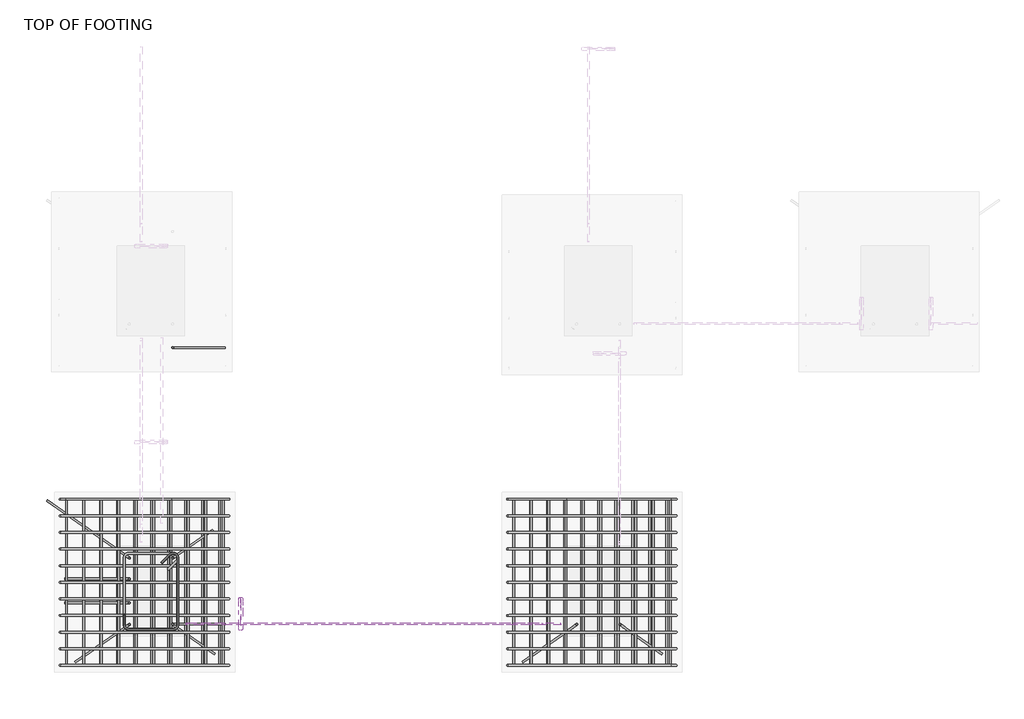
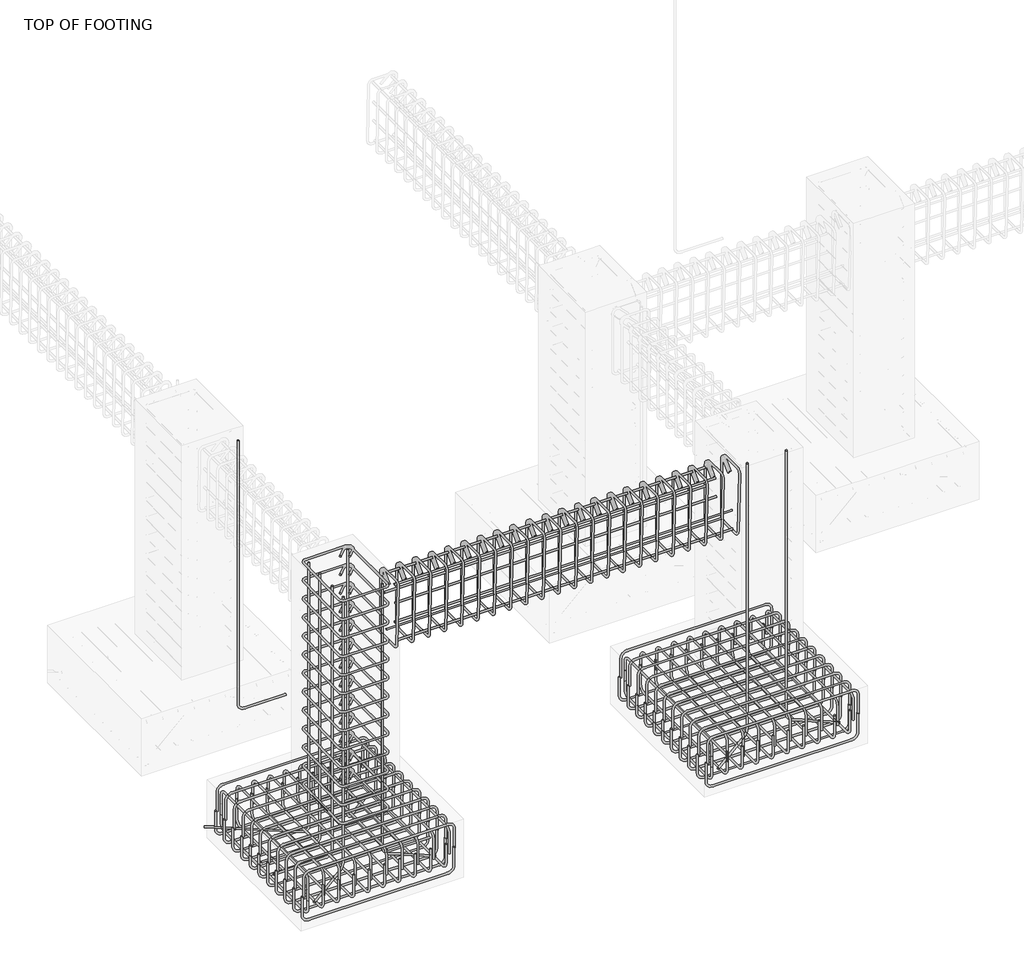
# One storey, part 2 of 17: 22 reinforcing bars.
"""IFC4 building model written with IfcOpenShell, lengths in millimetres."""

from ifc_helpers import new_model, si_unit, point, frame, origin, place, context, project, spatial, polyline, circle_curve, trimmed, segment, composite_curve, source, transform, mapped, element, save
from ifc_brep_helpers import swept_disk

model = new_model("IFC4")

# Units and contexts
model_context = context("Model", 3, world=origin())
ifc_project = project(units=[si_unit("LENGTHUNIT", "METRE", prefix="MILLI")], contexts=[model_context])

# Site, building, storey
site = spatial("IfcSite", under=ifc_project)
building = spatial("IfcBuilding", under=site)
storey = spatial("IfcBuildingStorey", under=building, Name="TOP OF FOOTING", Elevation=-1828.8)

# Reinforcing bars
placement = place(None, origin())
reinforcing_bar_shape = source(origin(), model_context, "Body", "SolidModel", [
    swept_disk(composite_curve([segment(polyline([(-2778.357124, -2320.8742842, -2051.4362487), (-2778.357124, -2320.8742842, -2198.7362487)]), True, "CONTINUOUS"), segment(trimmed(circle_curve(frame((-2824.707124, -2320.8742842, -2198.7362487), z_axis=(0.0, 1.0, 0.0), x_axis=(46.34999999999991, 0.0, 0.0)), 46.35), [point((-2778.357124, -2320.8742842, -2198.7362487))], [point((-2824.707124, -2320.8742842, -2245.0862487))], True, "CARTESIAN"), True, "CONTINUOUS"), segment(polyline([(-2824.707124, -2320.8742842, -2245.0862487), (-3850.0249485, -2320.8742842, -2245.0862487)]), True, "CONTINUOUS"), segment(trimmed(circle_curve(frame((-3850.0249485, -2320.8742842, -2198.7362487), z_axis=(0.0, 1.0, 0.0), x_axis=(0.0, 0.0, -46.34999999999991)), 46.35), [point((-3850.0249485, -2320.8742842, -2245.0862487))], [point((-3896.3749485, -2320.8742842, -2198.7362487))], True, "CARTESIAN"), True, "CONTINUOUS"), segment(polyline([(-3896.3749485, -2320.8742842, -2198.7362487), (-3896.3749485, -2320.8742842, -2051.4362487)]), True, "CONTINUOUS")], self_intersect=False), 6.35),
])
element("IfcReinforcingBar", 1, at=placement, inside=storey, context=model_context, shape_type="MappedRepresentation", body=[
    mapped(reinforcing_bar_shape, transform((0.0, 0.0, 0.0), x_axis=(1.0, 0.0, 0.0), y_axis=(0.0, 1.0, 0.0), z_axis=(0.0, 0.0, 1.0))),
    mapped(reinforcing_bar_shape, transform((0.0, -110.73, 0.0), x_axis=(1.0, 0.0, 0.0), y_axis=(0.0, 1.0, 0.0), z_axis=(0.0, 0.0, 1.0))),
    mapped(reinforcing_bar_shape, transform((0.0, -221.46, 0.0), x_axis=(1.0, 0.0, 0.0), y_axis=(0.0, 1.0, 0.0), z_axis=(0.0, 0.0, 1.0))),
    mapped(reinforcing_bar_shape, transform((0.0, -332.19, 0.0), x_axis=(1.0, 0.0, 0.0), y_axis=(0.0, 1.0, 0.0), z_axis=(0.0, 0.0, 1.0))),
    mapped(reinforcing_bar_shape, transform((0.0, -442.92, 0.0), x_axis=(1.0, 0.0, 0.0), y_axis=(0.0, 1.0, 0.0), z_axis=(0.0, 0.0, 1.0))),
    mapped(reinforcing_bar_shape, transform((0.0, -553.65, 0.0), x_axis=(1.0, 0.0, 0.0), y_axis=(0.0, 1.0, 0.0), z_axis=(0.0, 0.0, 1.0))),
    mapped(reinforcing_bar_shape, transform((0.0, -664.38, 0.0), x_axis=(1.0, 0.0, 0.0), y_axis=(0.0, 1.0, 0.0), z_axis=(0.0, 0.0, 1.0))),
    mapped(reinforcing_bar_shape, transform((0.0, -775.11, 0.0), x_axis=(1.0, 0.0, 0.0), y_axis=(0.0, 1.0, 0.0), z_axis=(0.0, 0.0, 1.0))),
    mapped(reinforcing_bar_shape, transform((0.0, -885.84, 0.0), x_axis=(1.0, 0.0, 0.0), y_axis=(0.0, 1.0, 0.0), z_axis=(0.0, 0.0, 1.0))),
    mapped(reinforcing_bar_shape, transform((0.0, -996.57, 0.0), x_axis=(1.0, 0.0, 0.0), y_axis=(0.0, 1.0, 0.0), z_axis=(0.0, 0.0, 1.0))),
    mapped(reinforcing_bar_shape, transform((0.0, -1107.3, 0.0), x_axis=(1.0, 0.0, 0.0), y_axis=(0.0, 1.0, 0.0), z_axis=(0.0, 0.0, 1.0))),
])
reinforcing_bar_2_shape = source(origin(), model_context, "Body", "SolidModel", [
    swept_disk(composite_curve([segment(polyline([(-3885.7112848, -2320.8742842, -2058.517229), (-3885.7112848, -2320.8742842, -1911.217229)]), True, "CONTINUOUS"), segment(trimmed(circle_curve(frame((-3839.3612848, -2320.8742842, -1911.217229), z_axis=(0.0, 1.0, 0.0), x_axis=(-46.350000000000364, 0.0, 0.0)), 46.35), [point((-3885.7112848, -2320.8742842, -1911.217229))], [point((-3839.3612848, -2320.8742842, -1864.867229))], True, "CARTESIAN"), True, "CONTINUOUS"), segment(polyline([(-3839.3612848, -2320.8742842, -1864.867229), (-2820.8048983, -2320.8742842, -1864.867229)]), True, "CONTINUOUS"), segment(trimmed(circle_curve(frame((-2820.8048983, -2320.8742842, -1911.217229), z_axis=(0.0, 1.0, 0.0), x_axis=(0.0, 0.0, 46.350000000000136)), 46.35), [point((-2820.8048983, -2320.8742842, -1864.867229))], [point((-2774.4548983, -2320.8742842, -1911.217229))], True, "CARTESIAN"), True, "CONTINUOUS"), segment(polyline([(-2774.4548983, -2320.8742842, -1911.217229), (-2774.4548983, -2320.8742842, -2058.517229)]), True, "CONTINUOUS")], self_intersect=False), 6.35),
])
element("IfcReinforcingBar", 2, at=placement, inside=storey, context=model_context, shape_type="MappedRepresentation", body=[
    mapped(reinforcing_bar_2_shape, transform((0.0, 0.0, 0.0), x_axis=(1.0, 0.0, 0.0), y_axis=(0.0, 1.0, 0.0), z_axis=(0.0, 0.0, 1.0))),
    mapped(reinforcing_bar_2_shape, transform((0.0, -110.73, 0.0), x_axis=(1.0, 0.0, 0.0), y_axis=(0.0, 1.0, 0.0), z_axis=(0.0, 0.0, 1.0))),
    mapped(reinforcing_bar_2_shape, transform((0.0, -221.46, 0.0), x_axis=(1.0, 0.0, 0.0), y_axis=(0.0, 1.0, 0.0), z_axis=(0.0, 0.0, 1.0))),
    mapped(reinforcing_bar_2_shape, transform((0.0, -332.19, 0.0), x_axis=(1.0, 0.0, 0.0), y_axis=(0.0, 1.0, 0.0), z_axis=(0.0, 0.0, 1.0))),
    mapped(reinforcing_bar_2_shape, transform((0.0, -442.92, 0.0), x_axis=(1.0, 0.0, 0.0), y_axis=(0.0, 1.0, 0.0), z_axis=(0.0, 0.0, 1.0))),
    mapped(reinforcing_bar_2_shape, transform((0.0, -553.65, 0.0), x_axis=(1.0, 0.0, 0.0), y_axis=(0.0, 1.0, 0.0), z_axis=(0.0, 0.0, 1.0))),
    mapped(reinforcing_bar_2_shape, transform((0.0, -664.38, 0.0), x_axis=(1.0, 0.0, 0.0), y_axis=(0.0, 1.0, 0.0), z_axis=(0.0, 0.0, 1.0))),
    mapped(reinforcing_bar_2_shape, transform((0.0, -775.11, 0.0), x_axis=(1.0, 0.0, 0.0), y_axis=(0.0, 1.0, 0.0), z_axis=(0.0, 0.0, 1.0))),
    mapped(reinforcing_bar_2_shape, transform((0.0, -885.84, 0.0), x_axis=(1.0, 0.0, 0.0), y_axis=(0.0, 1.0, 0.0), z_axis=(0.0, 0.0, 1.0))),
    mapped(reinforcing_bar_2_shape, transform((0.0, -996.57, 0.0), x_axis=(1.0, 0.0, 0.0), y_axis=(0.0, 1.0, 0.0), z_axis=(0.0, 0.0, 1.0))),
    mapped(reinforcing_bar_2_shape, transform((0.0, -1107.3, 0.0), x_axis=(1.0, 0.0, 0.0), y_axis=(0.0, 1.0, 0.0), z_axis=(0.0, 0.0, 1.0))),
])
reinforcing_bar_3_shape = source(origin(), model_context, "Body", "SolidModel", [
    swept_disk(composite_curve([segment(polyline([(-2811.4466034, -2320.8742842, -2093.0974099), (-2811.4466034, -2320.8742842, -1945.7974099)]), True, "CONTINUOUS"), segment(trimmed(circle_curve(frame((-2811.4466034, -2367.2242842, -1945.7974099), z_axis=(1.0, 0.0, 0.0), x_axis=(0.0, 46.34999999999991, 0.0)), 46.35), [point((-2811.4466034, -2320.8742842, -1945.7974099))], [point((-2811.4466034, -2367.2242842, -1899.4474099))], True, "CARTESIAN"), True, "CONTINUOUS"), segment(polyline([(-2811.4466034, -2367.2242842, -1899.4474099), (-2811.4466034, -3381.8242842, -1899.4474099)]), True, "CONTINUOUS"), segment(trimmed(circle_curve(frame((-2811.4466034, -3381.8242842, -1945.7974099), z_axis=(1.0, 0.0, 0.0), x_axis=(0.0, 0.0, 46.350000000000136)), 46.35), [point((-2811.4466034, -3381.8242842, -1899.4474099))], [point((-2811.4466034, -3428.1742842, -1945.7974099))], True, "CARTESIAN"), True, "CONTINUOUS"), segment(polyline([(-2811.4466034, -3428.1742842, -1945.7974099), (-2811.4466034, -3428.1742842, -2093.0974099)]), True, "CONTINUOUS")], self_intersect=False), 6.35),
])
element("IfcReinforcingBar", 3, at=placement, inside=storey, context=model_context, shape_type="MappedRepresentation", body=[
    mapped(reinforcing_bar_3_shape, transform((0.0, 0.0, 0.0), x_axis=(1.0, 0.0, 0.0), y_axis=(0.0, 1.0, 0.0), z_axis=(0.0, 0.0, 1.0))),
    mapped(reinforcing_bar_3_shape, transform((-115.9606781, 0.0, 0.0), x_axis=(1.0, 0.0, 0.0), y_axis=(0.0, 1.0, 0.0), z_axis=(0.0, 0.0, 1.0))),
    mapped(reinforcing_bar_3_shape, transform((-231.9213561, 0.0, 0.0), x_axis=(1.0, 0.0, 0.0), y_axis=(0.0, 1.0, 0.0), z_axis=(0.0, 0.0, 1.0))),
    mapped(reinforcing_bar_3_shape, transform((-347.8820342, 0.0, 0.0), x_axis=(1.0, 0.0, 0.0), y_axis=(0.0, 1.0, 0.0), z_axis=(0.0, 0.0, 1.0))),
    mapped(reinforcing_bar_3_shape, transform((-463.8427123, 0.0, 0.0), x_axis=(1.0, 0.0, 0.0), y_axis=(0.0, 1.0, 0.0), z_axis=(0.0, 0.0, 1.0))),
    mapped(reinforcing_bar_3_shape, transform((-579.8033904, 0.0, 0.0), x_axis=(1.0, 0.0, 0.0), y_axis=(0.0, 1.0, 0.0), z_axis=(0.0, 0.0, 1.0))),
    mapped(reinforcing_bar_3_shape, transform((-695.7640684, 0.0, 0.0), x_axis=(1.0, 0.0, 0.0), y_axis=(0.0, 1.0, 0.0), z_axis=(0.0, 0.0, 1.0))),
    mapped(reinforcing_bar_3_shape, transform((-811.7247465, 0.0, 0.0), x_axis=(1.0, 0.0, 0.0), y_axis=(0.0, 1.0, 0.0), z_axis=(0.0, 0.0, 1.0))),
    mapped(reinforcing_bar_3_shape, transform((-927.6854246, 0.0, 0.0), x_axis=(1.0, 0.0, 0.0), y_axis=(0.0, 1.0, 0.0), z_axis=(0.0, 0.0, 1.0))),
    mapped(reinforcing_bar_3_shape, transform((-1043.6461027, 0.0, 0.0), x_axis=(1.0, 0.0, 0.0), y_axis=(0.0, 1.0, 0.0), z_axis=(0.0, 0.0, 1.0))),
])
reinforcing_bar_4_shape = source(origin(), model_context, "Body", "SolidModel", [
    swept_disk(composite_curve([segment(polyline([(-3855.092706, -2320.8742842, -2009.4698822), (-3855.092706, -2320.8742842, -2156.7698822)]), True, "CONTINUOUS"), segment(trimmed(circle_curve(frame((-3855.092706, -2367.2242842, -2156.7698822), z_axis=(-1.0, 0.0, 0.0), x_axis=(0.0, 46.34999999999991, 0.0)), 46.35), [point((-3855.092706, -2320.8742842, -2156.7698822))], [point((-3855.092706, -2367.2242842, -2203.1198822))], True, "CARTESIAN"), True, "CONTINUOUS"), segment(polyline([(-3855.092706, -2367.2242842, -2203.1198822), (-3855.092706, -3381.8242842, -2203.1198822)]), True, "CONTINUOUS"), segment(trimmed(circle_curve(frame((-3855.092706, -3381.8242842, -2156.7698822), z_axis=(-1.0, 0.0, 0.0), x_axis=(0.0, 0.0, -46.34999999999991)), 46.35), [point((-3855.092706, -3381.8242842, -2203.1198822))], [point((-3855.092706, -3428.1742842, -2156.7698822))], True, "CARTESIAN"), True, "CONTINUOUS"), segment(polyline([(-3855.092706, -3428.1742842, -2156.7698822), (-3855.092706, -3428.1742842, -2009.4698822)]), True, "CONTINUOUS")], self_intersect=False), 6.35),
])
element("IfcReinforcingBar", 4, at=placement, inside=storey, context=model_context, shape_type="MappedRepresentation", body=[
    mapped(reinforcing_bar_4_shape, transform((0.0, 0.0, 0.0), x_axis=(1.0, 0.0, 0.0), y_axis=(0.0, 1.0, 0.0), z_axis=(0.0, 0.0, 1.0))),
    mapped(reinforcing_bar_4_shape, transform((113.1523491, 0.0, 0.0), x_axis=(1.0, 0.0, 0.0), y_axis=(0.0, 1.0, 0.0), z_axis=(0.0, 0.0, 1.0))),
    mapped(reinforcing_bar_4_shape, transform((226.3046983, 0.0, 0.0), x_axis=(1.0, 0.0, 0.0), y_axis=(0.0, 1.0, 0.0), z_axis=(0.0, 0.0, 1.0))),
    mapped(reinforcing_bar_4_shape, transform((339.4570474, 0.0, 0.0), x_axis=(1.0, 0.0, 0.0), y_axis=(0.0, 1.0, 0.0), z_axis=(0.0, 0.0, 1.0))),
    mapped(reinforcing_bar_4_shape, transform((452.6093966, 0.0, 0.0), x_axis=(1.0, 0.0, 0.0), y_axis=(0.0, 1.0, 0.0), z_axis=(0.0, 0.0, 1.0))),
    mapped(reinforcing_bar_4_shape, transform((565.7617457, 0.0, 0.0), x_axis=(1.0, 0.0, 0.0), y_axis=(0.0, 1.0, 0.0), z_axis=(0.0, 0.0, 1.0))),
    mapped(reinforcing_bar_4_shape, transform((678.9140949, 0.0, 0.0), x_axis=(1.0, 0.0, 0.0), y_axis=(0.0, 1.0, 0.0), z_axis=(0.0, 0.0, 1.0))),
    mapped(reinforcing_bar_4_shape, transform((792.066444, 0.0, 0.0), x_axis=(1.0, 0.0, 0.0), y_axis=(0.0, 1.0, 0.0), z_axis=(0.0, 0.0, 1.0))),
    mapped(reinforcing_bar_4_shape, transform((905.2187932, 0.0, 0.0), x_axis=(1.0, 0.0, 0.0), y_axis=(0.0, 1.0, 0.0), z_axis=(0.0, 0.0, 1.0))),
    mapped(reinforcing_bar_4_shape, transform((1018.3711423, 0.0, 0.0), x_axis=(1.0, 0.0, 0.0), y_axis=(0.0, 1.0, 0.0), z_axis=(0.0, 0.0, 1.0))),
])
reinforcing_bar_5_shape = source(origin(), model_context, "Body", "SolidModel", [
    swept_disk(composite_curve([segment(polyline([(199.2830257, -2320.8742842, -2051.4362487), (199.2830257, -2320.8742842, -2198.7362487)]), True, "CONTINUOUS"), segment(trimmed(circle_curve(frame((152.9330257, -2320.8742842, -2198.7362487), z_axis=(0.0, 1.0, 0.0), x_axis=(46.349999999999994, 0.0, 0.0)), 46.35), [point((199.2830257, -2320.8742842, -2198.7362487))], [point((152.9330257, -2320.8742842, -2245.0862487))], True, "CARTESIAN"), True, "CONTINUOUS"), segment(polyline([(152.9330257, -2320.8742842, -2245.0862487), (-872.3847988, -2320.8742842, -2245.0862487)]), True, "CONTINUOUS"), segment(trimmed(circle_curve(frame((-872.3847988, -2320.8742842, -2198.7362487), z_axis=(0.0, 1.0, 0.0), x_axis=(0.0, 0.0, -46.34999999999991)), 46.35), [point((-872.3847988, -2320.8742842, -2245.0862487))], [point((-918.7347988, -2320.8742842, -2198.7362487))], True, "CARTESIAN"), True, "CONTINUOUS"), segment(polyline([(-918.7347988, -2320.8742842, -2198.7362487), (-918.7347988, -2320.8742842, -2051.4362487)]), True, "CONTINUOUS")], self_intersect=False), 6.35),
])
element("IfcReinforcingBar", 5, at=placement, inside=storey, context=model_context, shape_type="MappedRepresentation", body=[
    mapped(reinforcing_bar_5_shape, transform((0.0, 0.0, 0.0), x_axis=(1.0, 0.0, 0.0), y_axis=(0.0, 1.0, 0.0), z_axis=(0.0, 0.0, 1.0))),
    mapped(reinforcing_bar_5_shape, transform((0.0, -110.73, 0.0), x_axis=(1.0, 0.0, 0.0), y_axis=(0.0, 1.0, 0.0), z_axis=(0.0, 0.0, 1.0))),
    mapped(reinforcing_bar_5_shape, transform((0.0, -221.46, 0.0), x_axis=(1.0, 0.0, 0.0), y_axis=(0.0, 1.0, 0.0), z_axis=(0.0, 0.0, 1.0))),
    mapped(reinforcing_bar_5_shape, transform((0.0, -332.19, 0.0), x_axis=(1.0, 0.0, 0.0), y_axis=(0.0, 1.0, 0.0), z_axis=(0.0, 0.0, 1.0))),
    mapped(reinforcing_bar_5_shape, transform((0.0, -442.92, 0.0), x_axis=(1.0, 0.0, 0.0), y_axis=(0.0, 1.0, 0.0), z_axis=(0.0, 0.0, 1.0))),
    mapped(reinforcing_bar_5_shape, transform((0.0, -553.65, 0.0), x_axis=(1.0, 0.0, 0.0), y_axis=(0.0, 1.0, 0.0), z_axis=(0.0, 0.0, 1.0))),
    mapped(reinforcing_bar_5_shape, transform((0.0, -664.38, 0.0), x_axis=(1.0, 0.0, 0.0), y_axis=(0.0, 1.0, 0.0), z_axis=(0.0, 0.0, 1.0))),
    mapped(reinforcing_bar_5_shape, transform((0.0, -775.11, 0.0), x_axis=(1.0, 0.0, 0.0), y_axis=(0.0, 1.0, 0.0), z_axis=(0.0, 0.0, 1.0))),
    mapped(reinforcing_bar_5_shape, transform((0.0, -885.84, 0.0), x_axis=(1.0, 0.0, 0.0), y_axis=(0.0, 1.0, 0.0), z_axis=(0.0, 0.0, 1.0))),
    mapped(reinforcing_bar_5_shape, transform((0.0, -996.57, 0.0), x_axis=(1.0, 0.0, 0.0), y_axis=(0.0, 1.0, 0.0), z_axis=(0.0, 0.0, 1.0))),
    mapped(reinforcing_bar_5_shape, transform((0.0, -1107.3, 0.0), x_axis=(1.0, 0.0, 0.0), y_axis=(0.0, 1.0, 0.0), z_axis=(0.0, 0.0, 1.0))),
])
reinforcing_bar_6_shape = source(origin(), model_context, "Body", "SolidModel", [
    swept_disk(composite_curve([segment(polyline([(-908.0711351, -2320.8742842, -2058.517229), (-908.0711351, -2320.8742842, -1911.217229)]), True, "CONTINUOUS"), segment(trimmed(circle_curve(frame((-861.7211351, -2320.8742842, -1911.217229), z_axis=(0.0, 1.0, 0.0), x_axis=(-46.35000000000002, 0.0, 0.0)), 46.35), [point((-908.0711351, -2320.8742842, -1911.217229))], [point((-861.7211351, -2320.8742842, -1864.867229))], True, "CARTESIAN"), True, "CONTINUOUS"), segment(polyline([(-861.7211351, -2320.8742842, -1864.867229), (156.8352514, -2320.8742842, -1864.867229)]), True, "CONTINUOUS"), segment(trimmed(circle_curve(frame((156.8352514, -2320.8742842, -1911.217229), z_axis=(0.0, 1.0, 0.0), x_axis=(0.0, 0.0, 46.350000000000136)), 46.35), [point((156.8352514, -2320.8742842, -1864.867229))], [point((203.1852514, -2320.8742842, -1911.217229))], True, "CARTESIAN"), True, "CONTINUOUS"), segment(polyline([(203.1852514, -2320.8742842, -1911.217229), (203.1852514, -2320.8742842, -2058.517229)]), True, "CONTINUOUS")], self_intersect=False), 6.35),
])
element("IfcReinforcingBar", 6, at=placement, inside=storey, context=model_context, shape_type="MappedRepresentation", body=[
    mapped(reinforcing_bar_6_shape, transform((0.0, 0.0, 0.0), x_axis=(1.0, 0.0, 0.0), y_axis=(0.0, 1.0, 0.0), z_axis=(0.0, 0.0, 1.0))),
    mapped(reinforcing_bar_6_shape, transform((0.0, -110.73, 0.0), x_axis=(1.0, 0.0, 0.0), y_axis=(0.0, 1.0, 0.0), z_axis=(0.0, 0.0, 1.0))),
    mapped(reinforcing_bar_6_shape, transform((0.0, -221.46, 0.0), x_axis=(1.0, 0.0, 0.0), y_axis=(0.0, 1.0, 0.0), z_axis=(0.0, 0.0, 1.0))),
    mapped(reinforcing_bar_6_shape, transform((0.0, -332.19, 0.0), x_axis=(1.0, 0.0, 0.0), y_axis=(0.0, 1.0, 0.0), z_axis=(0.0, 0.0, 1.0))),
    mapped(reinforcing_bar_6_shape, transform((0.0, -442.92, 0.0), x_axis=(1.0, 0.0, 0.0), y_axis=(0.0, 1.0, 0.0), z_axis=(0.0, 0.0, 1.0))),
    mapped(reinforcing_bar_6_shape, transform((0.0, -553.65, 0.0), x_axis=(1.0, 0.0, 0.0), y_axis=(0.0, 1.0, 0.0), z_axis=(0.0, 0.0, 1.0))),
    mapped(reinforcing_bar_6_shape, transform((0.0, -664.38, 0.0), x_axis=(1.0, 0.0, 0.0), y_axis=(0.0, 1.0, 0.0), z_axis=(0.0, 0.0, 1.0))),
    mapped(reinforcing_bar_6_shape, transform((0.0, -775.11, 0.0), x_axis=(1.0, 0.0, 0.0), y_axis=(0.0, 1.0, 0.0), z_axis=(0.0, 0.0, 1.0))),
    mapped(reinforcing_bar_6_shape, transform((0.0, -885.84, 0.0), x_axis=(1.0, 0.0, 0.0), y_axis=(0.0, 1.0, 0.0), z_axis=(0.0, 0.0, 1.0))),
    mapped(reinforcing_bar_6_shape, transform((0.0, -996.57, 0.0), x_axis=(1.0, 0.0, 0.0), y_axis=(0.0, 1.0, 0.0), z_axis=(0.0, 0.0, 1.0))),
    mapped(reinforcing_bar_6_shape, transform((0.0, -1107.3, 0.0), x_axis=(1.0, 0.0, 0.0), y_axis=(0.0, 1.0, 0.0), z_axis=(0.0, 0.0, 1.0))),
])
reinforcing_bar_7_shape = source(origin(), model_context, "Body", "SolidModel", [
    swept_disk(composite_curve([segment(polyline([(166.1935463, -2320.8742842, -2093.0974099), (166.1935463, -2320.8742842, -1945.7974099)]), True, "CONTINUOUS"), segment(trimmed(circle_curve(frame((166.1935463, -2367.2242842, -1945.7974099), z_axis=(1.0, 0.0, 0.0), x_axis=(0.0, 46.34999999999991, 0.0)), 46.35), [point((166.1935463, -2320.8742842, -1945.7974099))], [point((166.1935463, -2367.2242842, -1899.4474099))], True, "CARTESIAN"), True, "CONTINUOUS"), segment(polyline([(166.1935463, -2367.2242842, -1899.4474099), (166.1935463, -3381.8242842, -1899.4474099)]), True, "CONTINUOUS"), segment(trimmed(circle_curve(frame((166.1935463, -3381.8242842, -1945.7974099), z_axis=(1.0, 0.0, 0.0), x_axis=(0.0, 0.0, 46.350000000000136)), 46.35), [point((166.1935463, -3381.8242842, -1899.4474099))], [point((166.1935463, -3428.1742842, -1945.7974099))], True, "CARTESIAN"), True, "CONTINUOUS"), segment(polyline([(166.1935463, -3428.1742842, -1945.7974099), (166.1935463, -3428.1742842, -2093.0974099)]), True, "CONTINUOUS")], self_intersect=False), 6.35),
])
element("IfcReinforcingBar", 7, at=placement, inside=storey, context=model_context, shape_type="MappedRepresentation", body=[
    mapped(reinforcing_bar_7_shape, transform((0.0, 0.0, 0.0), x_axis=(1.0, 0.0, 0.0), y_axis=(0.0, 1.0, 0.0), z_axis=(0.0, 0.0, 1.0))),
    mapped(reinforcing_bar_7_shape, transform((-115.9606781, 0.0, 0.0), x_axis=(1.0, 0.0, 0.0), y_axis=(0.0, 1.0, 0.0), z_axis=(0.0, 0.0, 1.0))),
    mapped(reinforcing_bar_7_shape, transform((-231.9213561, 0.0, 0.0), x_axis=(1.0, 0.0, 0.0), y_axis=(0.0, 1.0, 0.0), z_axis=(0.0, 0.0, 1.0))),
    mapped(reinforcing_bar_7_shape, transform((-347.8820342, 0.0, 0.0), x_axis=(1.0, 0.0, 0.0), y_axis=(0.0, 1.0, 0.0), z_axis=(0.0, 0.0, 1.0))),
    mapped(reinforcing_bar_7_shape, transform((-463.8427123, 0.0, 0.0), x_axis=(1.0, 0.0, 0.0), y_axis=(0.0, 1.0, 0.0), z_axis=(0.0, 0.0, 1.0))),
    mapped(reinforcing_bar_7_shape, transform((-579.8033904, 0.0, 0.0), x_axis=(1.0, 0.0, 0.0), y_axis=(0.0, 1.0, 0.0), z_axis=(0.0, 0.0, 1.0))),
    mapped(reinforcing_bar_7_shape, transform((-695.7640684, 0.0, 0.0), x_axis=(1.0, 0.0, 0.0), y_axis=(0.0, 1.0, 0.0), z_axis=(0.0, 0.0, 1.0))),
    mapped(reinforcing_bar_7_shape, transform((-811.7247465, 0.0, 0.0), x_axis=(1.0, 0.0, 0.0), y_axis=(0.0, 1.0, 0.0), z_axis=(0.0, 0.0, 1.0))),
    mapped(reinforcing_bar_7_shape, transform((-927.6854246, 0.0, 0.0), x_axis=(1.0, 0.0, 0.0), y_axis=(0.0, 1.0, 0.0), z_axis=(0.0, 0.0, 1.0))),
    mapped(reinforcing_bar_7_shape, transform((-1043.6461027, 0.0, 0.0), x_axis=(1.0, 0.0, 0.0), y_axis=(0.0, 1.0, 0.0), z_axis=(0.0, 0.0, 1.0))),
])
reinforcing_bar_8_shape = source(origin(), model_context, "Body", "SolidModel", [
    swept_disk(composite_curve([segment(polyline([(-877.4525564, -2320.8742842, -2009.4698822), (-877.4525564, -2320.8742842, -2156.7698822)]), True, "CONTINUOUS"), segment(trimmed(circle_curve(frame((-877.4525564, -2367.2242842, -2156.7698822), z_axis=(-1.0, 0.0, 0.0), x_axis=(0.0, 46.34999999999991, 0.0)), 46.35), [point((-877.4525564, -2320.8742842, -2156.7698822))], [point((-877.4525564, -2367.2242842, -2203.1198822))], True, "CARTESIAN"), True, "CONTINUOUS"), segment(polyline([(-877.4525564, -2367.2242842, -2203.1198822), (-877.4525564, -3381.8242842, -2203.1198822)]), True, "CONTINUOUS"), segment(trimmed(circle_curve(frame((-877.4525564, -3381.8242842, -2156.7698822), z_axis=(-1.0, 0.0, 0.0), x_axis=(0.0, 0.0, -46.34999999999991)), 46.35), [point((-877.4525564, -3381.8242842, -2203.1198822))], [point((-877.4525564, -3428.1742842, -2156.7698822))], True, "CARTESIAN"), True, "CONTINUOUS"), segment(polyline([(-877.4525564, -3428.1742842, -2156.7698822), (-877.4525564, -3428.1742842, -2009.4698822)]), True, "CONTINUOUS")], self_intersect=False), 6.35),
])
element("IfcReinforcingBar", 8, at=placement, inside=storey, context=model_context, shape_type="MappedRepresentation", body=[
    mapped(reinforcing_bar_8_shape, transform((0.0, 0.0, 0.0), x_axis=(1.0, 0.0, 0.0), y_axis=(0.0, 1.0, 0.0), z_axis=(0.0, 0.0, 1.0))),
    mapped(reinforcing_bar_8_shape, transform((113.1523491, 0.0, 0.0), x_axis=(1.0, 0.0, 0.0), y_axis=(0.0, 1.0, 0.0), z_axis=(0.0, 0.0, 1.0))),
    mapped(reinforcing_bar_8_shape, transform((226.3046983, 0.0, 0.0), x_axis=(1.0, 0.0, 0.0), y_axis=(0.0, 1.0, 0.0), z_axis=(0.0, 0.0, 1.0))),
    mapped(reinforcing_bar_8_shape, transform((339.4570474, 0.0, 0.0), x_axis=(1.0, 0.0, 0.0), y_axis=(0.0, 1.0, 0.0), z_axis=(0.0, 0.0, 1.0))),
    mapped(reinforcing_bar_8_shape, transform((452.6093966, 0.0, 0.0), x_axis=(1.0, 0.0, 0.0), y_axis=(0.0, 1.0, 0.0), z_axis=(0.0, 0.0, 1.0))),
    mapped(reinforcing_bar_8_shape, transform((565.7617457, 0.0, 0.0), x_axis=(1.0, 0.0, 0.0), y_axis=(0.0, 1.0, 0.0), z_axis=(0.0, 0.0, 1.0))),
    mapped(reinforcing_bar_8_shape, transform((678.9140949, 0.0, 0.0), x_axis=(1.0, 0.0, 0.0), y_axis=(0.0, 1.0, 0.0), z_axis=(0.0, 0.0, 1.0))),
    mapped(reinforcing_bar_8_shape, transform((792.066444, 0.0, 0.0), x_axis=(1.0, 0.0, 0.0), y_axis=(0.0, 1.0, 0.0), z_axis=(0.0, 0.0, 1.0))),
    mapped(reinforcing_bar_8_shape, transform((905.2187932, 0.0, 0.0), x_axis=(1.0, 0.0, 0.0), y_axis=(0.0, 1.0, 0.0), z_axis=(0.0, 0.0, 1.0))),
    mapped(reinforcing_bar_8_shape, transform((1018.3711423, 0.0, 0.0), x_axis=(1.0, 0.0, 0.0), y_axis=(0.0, 1.0, 0.0), z_axis=(0.0, 0.0, 1.0))),
])
reinforcing_bar_9_shape = source(origin(), model_context, "Body", "SolidModel", [
    swept_disk(composite_curve([segment(polyline([(-3222.6184845, -2745.8000495, -46.35), (-3166.8749216, -2690.0564866, -46.35)]), True, "CONTINUOUS"), segment(trimmed(circle_curve(frame((-3144.707124, -2712.2242842, -46.35), z_axis=(0.0, 0.0, -1.0), x_axis=(-22.167797600000085, 22.167797600000085, 0.0)), 31.35), [point((-3166.8749216, -2690.0564866, -46.35))], [point((-3113.357124, -2712.2242842, -46.35))], True, "CARTESIAN"), True, "CONTINUOUS"), segment(polyline([(-3113.357124, -2712.2242842, -46.35), (-3113.357124, -3156.8242842, -46.35)]), True, "CONTINUOUS"), segment(trimmed(circle_curve(frame((-3144.707124, -3156.8242842, -46.35), z_axis=(0.0, 0.0, -1.0), x_axis=(31.34999999999991, 0.0, 0.0)), 31.35), [point((-3113.357124, -3156.8242842, -46.35))], [point((-3144.707124, -3188.1742842, -46.35))], True, "CARTESIAN"), True, "CONTINUOUS"), segment(polyline([(-3144.707124, -3188.1742842, -46.35), (-3439.307124, -3188.1742842, -46.35)]), True, "CONTINUOUS"), segment(trimmed(circle_curve(frame((-3439.307124, -3156.8341035, -45.5654144), z_axis=(0.0, 0.025026655153786343, -0.9996867842138424), x_axis=(0.0, -31.34018070000002, -0.7845855999999998)), 31.35), [point((-3439.307124, -3188.1742842, -46.35))], [point((-3470.657124, -3156.8341035, -45.5654144))], True, "CARTESIAN"), True, "CONTINUOUS"), segment(polyline([(-3470.657124, -3156.8341035, -45.5654144), (-3470.657124, -2712.2144649, -34.4345856)]), True, "CONTINUOUS"), segment(trimmed(circle_curve(frame((-3439.307124, -2712.2144649, -34.4345856), z_axis=(0.0, 0.025026655153786343, -0.9996867842138424), x_axis=(-31.34999999999991, 0.0, 0.0)), 31.35), [point((-3470.657124, -2712.2144649, -34.4345856))], [point((-3439.307124, -2680.8742842, -33.65))], True, "CARTESIAN"), True, "CONTINUOUS"), segment(polyline([(-3439.307124, -2680.8742842, -33.65), (-3144.707124, -2680.8742842, -33.65)]), True, "CONTINUOUS"), segment(trimmed(circle_curve(frame((-3144.707124, -2712.2242842, -33.65), z_axis=(0.0, 0.0, -1.0), x_axis=(0.0, 31.34999999999991, 0.0)), 31.35), [point((-3144.707124, -2680.8742842, -33.65))], [point((-3122.5393264, -2734.3920818, -33.65))], True, "CARTESIAN"), True, "CONTINUOUS"), segment(polyline([(-3122.5393264, -2734.3920818, -33.65), (-3178.2828893, -2790.1356447, -33.65)]), True, "CONTINUOUS")], self_intersect=False), 6.35),
])
element("IfcReinforcingBar", 9, at=placement, inside=storey, context=model_context, shape_type="MappedRepresentation", body=[
    mapped(reinforcing_bar_9_shape, transform((0.0, 0.0, 0.0), x_axis=(1.0, 0.0, 0.0), y_axis=(0.0, 1.0, 0.0), z_axis=(0.0, 0.0, 1.0))),
    mapped(reinforcing_bar_9_shape, transform((0.0, 0.0, -144.675), x_axis=(1.0, 0.0, 0.0), y_axis=(0.0, 1.0, 0.0), z_axis=(0.0, 0.0, 1.0))),
    mapped(reinforcing_bar_9_shape, transform((0.0, 0.0, -289.35), x_axis=(1.0, 0.0, 0.0), y_axis=(0.0, 1.0, 0.0), z_axis=(0.0, 0.0, 1.0))),
    mapped(reinforcing_bar_9_shape, transform((0.0, 0.0, -434.025), x_axis=(1.0, 0.0, 0.0), y_axis=(0.0, 1.0, 0.0), z_axis=(0.0, 0.0, 1.0))),
    mapped(reinforcing_bar_9_shape, transform((0.0, 0.0, -578.7), x_axis=(1.0, 0.0, 0.0), y_axis=(0.0, 1.0, 0.0), z_axis=(0.0, 0.0, 1.0))),
    mapped(reinforcing_bar_9_shape, transform((0.0, 0.0, -723.375), x_axis=(1.0, 0.0, 0.0), y_axis=(0.0, 1.0, 0.0), z_axis=(0.0, 0.0, 1.0))),
    mapped(reinforcing_bar_9_shape, transform((0.0, 0.0, -868.05), x_axis=(1.0, 0.0, 0.0), y_axis=(0.0, 1.0, 0.0), z_axis=(0.0, 0.0, 1.0))),
    mapped(reinforcing_bar_9_shape, transform((0.0, 0.0, -1012.725), x_axis=(1.0, 0.0, 0.0), y_axis=(0.0, 1.0, 0.0), z_axis=(0.0, 0.0, 1.0))),
    mapped(reinforcing_bar_9_shape, transform((0.0, 0.0, -1157.4), x_axis=(1.0, 0.0, 0.0), y_axis=(0.0, 1.0, 0.0), z_axis=(0.0, 0.0, 1.0))),
    mapped(reinforcing_bar_9_shape, transform((0.0, 0.0, -1302.075), x_axis=(1.0, 0.0, 0.0), y_axis=(0.0, 1.0, 0.0), z_axis=(0.0, 0.0, 1.0))),
    mapped(reinforcing_bar_9_shape, transform((0.0, 0.0, -1446.75), x_axis=(1.0, 0.0, 0.0), y_axis=(0.0, 1.0, 0.0), z_axis=(0.0, 0.0, 1.0))),
    mapped(reinforcing_bar_9_shape, transform((0.0, 0.0, -1591.425), x_axis=(1.0, 0.0, 0.0), y_axis=(0.0, 1.0, 0.0), z_axis=(0.0, 0.0, 1.0))),
    mapped(reinforcing_bar_9_shape, transform((0.0, 0.0, -1736.1), x_axis=(1.0, 0.0, 0.0), y_axis=(0.0, 1.0, 0.0), z_axis=(0.0, 0.0, 1.0))),
])
reinforcing_bar_10_shape = source(origin(), model_context, "Body", "SolidModel", [
    swept_disk(composite_curve([segment(polyline([(-3147.7427136, -3152.6310005, -40.0), (-3147.7427136, -3152.6310005, -2094.5391135)]), True, "CONTINUOUS"), segment(trimmed(circle_curve(frame((-3101.3927136, -3152.6310005, -2094.5391135), z_axis=(0.0, -1.0, 0.0), x_axis=(-46.34999999999991, 0.0, 0.0)), 46.35), [point((-3147.7427136, -3152.6310005, -2094.5391135))], [point((-3101.3927136, -3152.6310005, -2140.8891135))], True, "CARTESIAN"), True, "CONTINUOUS"), segment(polyline([(-3101.3927136, -3152.6310005, -2140.8891135), (-2797.6608063, -3152.6310005, -2140.8891135)]), True, "CONTINUOUS")], self_intersect=False), 6.35),
])
element("IfcReinforcingBar", 10, at=placement, inside=storey, context=model_context, shape_type="MappedRepresentation", body=[
    mapped(reinforcing_bar_10_shape, transform((0.0, 0.0, 0.0), x_axis=(1.0, 0.0, 0.0), y_axis=(0.0, 1.0, 0.0), z_axis=(0.0, 0.0, 1.0))),
    mapped(reinforcing_bar_10_shape, transform((0.0, 1840.7260472, 0.0), x_axis=(1.0, 0.0, 0.0), y_axis=(0.0, 1.0, 0.0), z_axis=(0.0, 0.0, 1.0))),
])
element("IfcReinforcingBar", 11, at=placement, inside=storey, context=model_context, shape_type="SolidModel", body=[
    swept_disk(composite_curve([segment(polyline([(-3147.7427136, -2713.5742842, -40.0), (-3147.7427136, -2713.5742842, -2094.5391135)]), True, "CONTINUOUS"), segment(trimmed(circle_curve(frame((-3109.7750164, -2686.9890164, -2094.5391135), z_axis=(0.5735764363510363, -0.8191520442889988, 0.0), x_axis=(-37.9676972000002, -26.58526780000011, 0.0)), 46.35), [point((-3147.7427136, -2713.5742842, -2094.5391135))], [point((-3109.7750164, -2686.9890164, -2140.8891135))], True, "CARTESIAN"), True, "CONTINUOUS"), segment(polyline([(-3109.7750164, -2686.9890164, -2140.8891135), (-2881.4249234, -2527.0965599, -2140.8891135)]), True, "CONTINUOUS")], self_intersect=False), 6.35),
])
element("IfcReinforcingBar", 12, at=placement, inside=storey, context=model_context, shape_type="SolidModel", body=[
    swept_disk(composite_curve([segment(polyline([(-3436.2715343, -2713.5742842, -40.0), (-3436.2715343, -2713.5742842, -2094.5391135)]), True, "CONTINUOUS"), segment(trimmed(circle_curve(frame((-3474.2392316, -2686.9890164, -2094.5391135), z_axis=(0.5735764363510419, 0.8191520442889948, 0.0), x_axis=(37.967697300000054, -26.58526780000011, 0.0)), 46.35), [point((-3436.2715343, -2713.5742842, -2094.5391135))], [point((-3474.2392316, -2686.9890164, -2140.8891135))], True, "CARTESIAN"), True, "CONTINUOUS"), segment(polyline([(-3474.2392316, -2686.9890164, -2140.8891135), (-3984.3116072, -2329.8324939, -2140.8891135)]), True, "CONTINUOUS")], self_intersect=False), 6.35),
])
element("IfcReinforcingBar", 13, at=placement, inside=storey, context=model_context, shape_type="SolidModel", body=[
    swept_disk(composite_curve([segment(polyline([(-3147.7427136, -3155.4742842, -40.0), (-3147.7427136, -3155.4742842, -2094.5391135)]), True, "CONTINUOUS"), segment(trimmed(circle_curve(frame((-3109.7750164, -3182.059552, -2094.5391135), z_axis=(-0.5735764363510363, -0.8191520442889988, 0.0), x_axis=(-37.9676972000002, 26.58526780000011, 0.0)), 46.35), [point((-3147.7427136, -3155.4742842, -2094.5391135))], [point((-3109.7750164, -3182.059552, -2140.8891135))], True, "CARTESIAN"), True, "CONTINUOUS"), segment(polyline([(-3109.7750164, -3182.059552, -2140.8891135), (-2868.2063218, -3351.207773, -2140.8891135)]), True, "CONTINUOUS")], self_intersect=False), 6.35),
])
element("IfcReinforcingBar", 14, at=placement, inside=storey, context=model_context, shape_type="SolidModel", body=[
    swept_disk(composite_curve([segment(polyline([(-3436.2715343, -3155.4742842, -40.0), (-3436.2715343, -3155.4742842, -2094.5391135)]), True, "CONTINUOUS"), segment(trimmed(circle_curve(frame((-3474.2392316, -3182.059552, -2094.5391135), z_axis=(-0.5735764363510419, 0.8191520442889948, 0.0), x_axis=(37.967697300000054, 26.58526780000011, 0.0)), 46.35), [point((-3436.2715343, -3155.4742842, -2094.5391135))], [point((-3474.2392316, -3182.059552, -2140.8891135))], True, "CARTESIAN"), True, "CONTINUOUS"), segment(polyline([(-3474.2392316, -3182.059552, -2140.8891135), (-3795.8079262, -3407.224376, -2140.8891135)]), True, "CONTINUOUS")], self_intersect=False), 6.35),
])
reinforcing_bar_11_shape = source(origin(), model_context, "Body", "SolidModel", [
    swept_disk(composite_curve([segment(polyline([(-3436.2715343, -2852.6310005, -40.0), (-3436.2715343, -2852.6310005, -2094.5391135)]), True, "CONTINUOUS"), segment(trimmed(circle_curve(frame((-3482.6215343, -2852.6310005, -2094.5391135), z_axis=(0.0, 1.0, 0.0), x_axis=(46.34999999999991, 0.0, 0.0)), 46.35), [point((-3436.2715343, -2852.6310005, -2094.5391135))], [point((-3482.6215343, -2852.6310005, -2140.8891135))], True, "CARTESIAN"), True, "CONTINUOUS"), segment(polyline([(-3482.6215343, -2852.6310005, -2140.8891135), (-3866.3534417, -2852.6310005, -2140.8891135)]), True, "CONTINUOUS")], self_intersect=False), 6.35),
])
element("IfcReinforcingBar", 15, at=placement, inside=storey, context=model_context, shape_type="MappedRepresentation", body=[
    mapped(reinforcing_bar_11_shape, transform((0.0, 0.0, 0.0), x_axis=(1.0, 0.0, 0.0), y_axis=(0.0, 1.0, 0.0), z_axis=(0.0, 0.0, 1.0))),
    mapped(reinforcing_bar_11_shape, transform((0.0, -159.2739528, 0.0), x_axis=(1.0, 0.0, 0.0), y_axis=(0.0, 1.0, 0.0), z_axis=(0.0, 0.0, 1.0))),
])
element("IfcReinforcingBar", 16, at=placement, inside=storey, context=model_context, shape_type="SolidModel", body=[
    swept_disk(composite_curve([segment(polyline([(-170.102564, -3155.4742842, -40.0), (-170.102564, -3155.4742842, -2094.5391135)]), True, "CONTINUOUS"), segment(trimmed(circle_curve(frame((-132.1348667, -3182.059552, -2094.5391135), z_axis=(-0.5735764363510363, -0.8191520442889988, 0.0), x_axis=(-37.9676973, 26.58526780000011, 0.0)), 46.35), [point((-170.102564, -3155.4742842, -2094.5391135))], [point((-132.1348667, -3182.059552, -2140.8891135))], True, "CARTESIAN"), True, "CONTINUOUS"), segment(polyline([(-132.1348667, -3182.059552, -2140.8891135), (109.4338279, -3351.207773, -2140.8891135)]), True, "CONTINUOUS")], self_intersect=False), 6.35),
])
element("IfcReinforcingBar", 17, at=placement, inside=storey, context=model_context, shape_type="SolidModel", body=[
    swept_disk(composite_curve([segment(polyline([(-458.6313847, -3155.4742842, -40.0), (-458.6313847, -3155.4742842, -2094.5391135)]), True, "CONTINUOUS"), segment(trimmed(circle_curve(frame((-496.5990819, -3182.059552, -2094.5391135), z_axis=(-0.5735764363510419, 0.8191520442889948, 0.0), x_axis=(37.967697199999975, 26.58526780000011, 0.0)), 46.35), [point((-458.6313847, -3155.4742842, -2094.5391135))], [point((-496.5990819, -3182.059552, -2140.8891135))], True, "CARTESIAN"), True, "CONTINUOUS"), segment(polyline([(-496.5990819, -3182.059552, -2140.8891135), (-818.1677765, -3407.224376, -2140.8891135)]), True, "CONTINUOUS")], self_intersect=False), 6.35),
])
reinforcing_bar_12_shape = source(origin(), model_context, "Body", "SolidModel", [
    swept_disk(composite_curve([segment(polyline([(-545.7169743, -3090.1356447, -111.2757654), (-545.7169743, -3034.3920818, -55.5322024)]), True, "CONTINUOUS"), segment(trimmed(circle_curve(frame((-545.7169743, -3012.2242842, -77.7), z_axis=(-1.0, 0.0, 0.0), x_axis=(0.0, -22.167797600000085, 22.1677976)), 31.35), [point((-545.7169743, -3034.3920818, -55.5322024))], [point((-545.7169743, -2980.8742842, -77.7))], True, "CARTESIAN"), True, "CONTINUOUS"), segment(polyline([(-545.7169743, -2980.8742842, -77.7), (-545.7169743, -2980.8742842, -522.3)]), True, "CONTINUOUS"), segment(trimmed(circle_curve(frame((-545.7169743, -3012.2242842, -522.3), z_axis=(-1.0, 0.0, 0.0), x_axis=(0.0, 31.34999999999991, 0.0)), 31.35), [point((-545.7169743, -2980.8742842, -522.3))], [point((-545.7169743, -3012.2242842, -553.65))], True, "CARTESIAN"), True, "CONTINUOUS"), segment(polyline([(-545.7169743, -3012.2242842, -553.65), (-545.7169743, -3156.8242842, -553.65)]), True, "CONTINUOUS"), segment(trimmed(circle_curve(frame((-544.9323887, -3156.8242842, -522.3098193), z_axis=(-0.9996867842138424, 0.0, 0.025026655153786322), x_axis=(-0.7845855999999003, 0.0, -31.34018070000002)), 31.35), [point((-545.7169743, -3156.8242842, -553.65))], [point((-544.9323887, -3188.1742842, -522.3098193))], True, "CARTESIAN"), True, "CONTINUOUS"), segment(polyline([(-544.9323887, -3188.1742842, -522.3098193), (-533.80156, -3188.1742842, -77.6901807)]), True, "CONTINUOUS"), segment(trimmed(circle_curve(frame((-533.80156, -3156.8242842, -77.6901807), z_axis=(-0.9996867842138424, 0.0, 0.025026655153786322), x_axis=(0.0, -31.34999999999991, 0.0)), 31.35), [point((-533.80156, -3188.1742842, -77.6901807))], [point((-533.0169743, -3156.8242842, -46.35))], True, "CARTESIAN"), True, "CONTINUOUS"), segment(polyline([(-533.0169743, -3156.8242842, -46.35), (-533.0169743, -3012.2242842, -46.35)]), True, "CONTINUOUS"), segment(trimmed(circle_curve(frame((-533.0169743, -3012.2242842, -77.7), z_axis=(-1.0, 0.0, 0.0), x_axis=(0.0, 0.0, 31.35)), 31.35), [point((-533.0169743, -3012.2242842, -46.35))], [point((-533.0169743, -2990.0564866, -99.8677976))], True, "CARTESIAN"), True, "CONTINUOUS"), segment(polyline([(-533.0169743, -2990.0564866, -99.8677976), (-533.0169743, -3045.8000495, -155.6113605)]), True, "CONTINUOUS")], self_intersect=False), 6.35),
])
element("IfcReinforcingBar", 18, at=placement, inside=storey, context=model_context, shape_type="MappedRepresentation", body=[
    mapped(reinforcing_bar_12_shape, transform((0.0, 0.0, 0.0), x_axis=(1.0, 0.0, 0.0), y_axis=(0.0, 1.0, 0.0), z_axis=(0.0, 0.0, 1.0))),
    mapped(reinforcing_bar_12_shape, transform((-119.7590547, 0.0, 0.0), x_axis=(1.0, 0.0, 0.0), y_axis=(0.0, 1.0, 0.0), z_axis=(0.0, 0.0, 1.0))),
    mapped(reinforcing_bar_12_shape, transform((-239.5181095, 0.0, 0.0), x_axis=(1.0, 0.0, 0.0), y_axis=(0.0, 1.0, 0.0), z_axis=(0.0, 0.0, 1.0))),
    mapped(reinforcing_bar_12_shape, transform((-359.2771642, 0.0, 0.0), x_axis=(1.0, 0.0, 0.0), y_axis=(0.0, 1.0, 0.0), z_axis=(0.0, 0.0, 1.0))),
    mapped(reinforcing_bar_12_shape, transform((-479.036219, 0.0, 0.0), x_axis=(1.0, 0.0, 0.0), y_axis=(0.0, 1.0, 0.0), z_axis=(0.0, 0.0, 1.0))),
    mapped(reinforcing_bar_12_shape, transform((-598.7952737, 0.0, 0.0), x_axis=(1.0, 0.0, 0.0), y_axis=(0.0, 1.0, 0.0), z_axis=(0.0, 0.0, 1.0))),
    mapped(reinforcing_bar_12_shape, transform((-718.5543285, 0.0, 0.0), x_axis=(1.0, 0.0, 0.0), y_axis=(0.0, 1.0, 0.0), z_axis=(0.0, 0.0, 1.0))),
    mapped(reinforcing_bar_12_shape, transform((-838.3133832, 0.0, 0.0), x_axis=(1.0, 0.0, 0.0), y_axis=(0.0, 1.0, 0.0), z_axis=(0.0, 0.0, 1.0))),
    mapped(reinforcing_bar_12_shape, transform((-958.072438, 0.0, 0.0), x_axis=(1.0, 0.0, 0.0), y_axis=(0.0, 1.0, 0.0), z_axis=(0.0, 0.0, 1.0))),
    mapped(reinforcing_bar_12_shape, transform((-1077.8314927, 0.0, 0.0), x_axis=(1.0, 0.0, 0.0), y_axis=(0.0, 1.0, 0.0), z_axis=(0.0, 0.0, 1.0))),
    mapped(reinforcing_bar_12_shape, transform((-1197.5905475, 0.0, 0.0), x_axis=(1.0, 0.0, 0.0), y_axis=(0.0, 1.0, 0.0), z_axis=(0.0, 0.0, 1.0))),
    mapped(reinforcing_bar_12_shape, transform((-1317.3496022, 0.0, 0.0), x_axis=(1.0, 0.0, 0.0), y_axis=(0.0, 1.0, 0.0), z_axis=(0.0, 0.0, 1.0))),
    mapped(reinforcing_bar_12_shape, transform((-1437.1086569, 0.0, 0.0), x_axis=(1.0, 0.0, 0.0), y_axis=(0.0, 1.0, 0.0), z_axis=(0.0, 0.0, 1.0))),
    mapped(reinforcing_bar_12_shape, transform((-1556.8677117, 0.0, 0.0), x_axis=(1.0, 0.0, 0.0), y_axis=(0.0, 1.0, 0.0), z_axis=(0.0, 0.0, 1.0))),
    mapped(reinforcing_bar_12_shape, transform((-1676.6267664, 0.0, 0.0), x_axis=(1.0, 0.0, 0.0), y_axis=(0.0, 1.0, 0.0), z_axis=(0.0, 0.0, 1.0))),
    mapped(reinforcing_bar_12_shape, transform((-1796.3858212, 0.0, 0.0), x_axis=(1.0, 0.0, 0.0), y_axis=(0.0, 1.0, 0.0), z_axis=(0.0, 0.0, 1.0))),
    mapped(reinforcing_bar_12_shape, transform((-1916.1448759, 0.0, 0.0), x_axis=(1.0, 0.0, 0.0), y_axis=(0.0, 1.0, 0.0), z_axis=(0.0, 0.0, 1.0))),
    mapped(reinforcing_bar_12_shape, transform((-2035.9039307, 0.0, 0.0), x_axis=(1.0, 0.0, 0.0), y_axis=(0.0, 1.0, 0.0), z_axis=(0.0, 0.0, 1.0))),
    mapped(reinforcing_bar_12_shape, transform((-2155.6629854, 0.0, 0.0), x_axis=(1.0, 0.0, 0.0), y_axis=(0.0, 1.0, 0.0), z_axis=(0.0, 0.0, 1.0))),
    mapped(reinforcing_bar_12_shape, transform((-2275.4220402, 0.0, 0.0), x_axis=(1.0, 0.0, 0.0), y_axis=(0.0, 1.0, 0.0), z_axis=(0.0, 0.0, 1.0))),
    mapped(reinforcing_bar_12_shape, transform((-2395.1810949, 0.0, 0.0), x_axis=(1.0, 0.0, 0.0), y_axis=(0.0, 1.0, 0.0), z_axis=(0.0, 0.0, 1.0))),
    mapped(reinforcing_bar_12_shape, transform((-2514.9401497, 0.0, 0.0), x_axis=(1.0, 0.0, 0.0), y_axis=(0.0, 1.0, 0.0), z_axis=(0.0, 0.0, 1.0))),
])
reinforcing_bar_13_shape = source(origin(), model_context, "Body", "SolidModel", [
    swept_disk(composite_curve([segment(polyline([(-690.2190947, -3150.3631867, -77.7), (-3056.7652893, -3150.3631867, -77.7)]), True, "CONTINUOUS")], self_intersect=False), 6.35),
])
element("IfcReinforcingBar", 19, at=placement, inside=storey, context=model_context, shape_type="MappedRepresentation", body=[
    mapped(reinforcing_bar_13_shape, transform((0.0, 0.0, 0.0), x_axis=(1.0, 0.0, 0.0), y_axis=(0.0, 1.0, 0.0), z_axis=(0.0, 0.0, 1.0))),
    mapped(reinforcing_bar_13_shape, transform((0.0, 137.266313, 0.0), x_axis=(1.0, 0.0, 0.0), y_axis=(0.0, 1.0, 0.0), z_axis=(0.0, 0.0, 1.0))),
])
reinforcing_bar_14_shape = source(origin(), model_context, "Body", "SolidModel", [
    swept_disk(composite_curve([segment(polyline([(-564.7818881, -3150.3631867, -517.7), (-3036.8338373, -3150.3631867, -517.7)]), True, "CONTINUOUS")], self_intersect=False), 6.35),
])
element("IfcReinforcingBar", 20, at=placement, inside=storey, context=model_context, shape_type="MappedRepresentation", body=[
    mapped(reinforcing_bar_14_shape, transform((0.0, 0.0, 0.0), x_axis=(1.0, 0.0, 0.0), y_axis=(0.0, 1.0, 0.0), z_axis=(0.0, 0.0, 1.0))),
    mapped(reinforcing_bar_14_shape, transform((0.0, 137.266313, 0.0), x_axis=(1.0, 0.0, 0.0), y_axis=(0.0, 1.0, 0.0), z_axis=(0.0, 0.0, 1.0))),
])
reinforcing_bar_15_shape = source(origin(), model_context, "Body", "SolidModel", [
    swept_disk(composite_curve([segment(polyline([(-684.0716824, -3150.3631867, -224.3666667), (-3052.5461064, -3150.3631867, -224.3666667)]), True, "CONTINUOUS")], self_intersect=False), 6.35),
])
element("IfcReinforcingBar", 21, at=placement, inside=storey, context=model_context, shape_type="MappedRepresentation", body=[
    mapped(reinforcing_bar_15_shape, transform((0.0, 0.0, 0.0), x_axis=(1.0, 0.0, 0.0), y_axis=(0.0, 1.0, 0.0), z_axis=(0.0, 0.0, 1.0))),
    mapped(reinforcing_bar_15_shape, transform((0.0, 137.266313, 0.0), x_axis=(1.0, 0.0, 0.0), y_axis=(0.0, 1.0, 0.0), z_axis=(0.0, 0.0, 1.0))),
])
element("IfcReinforcingBar", 22, at=placement, inside=storey, context=model_context, shape_type="SolidModel", body=[
    swept_disk(composite_curve([segment(polyline([(-568.1551192, -3150.3631867, -371.0333333), (-3054.6556979, -3150.3631867, -371.0333333)]), True, "CONTINUOUS")], self_intersect=False), 6.35),
])

save(model, "model.ifc")

# Revit data of these elements
# Elements 1, 2, 3, 4, 5, 6, 7, 8, 9, 10, 11, 12, 13, 14, 15, 16, 17, 18, 19, 20, 21, 22 (IfcReinforcingBar)
#   Phase Created = New Construction
